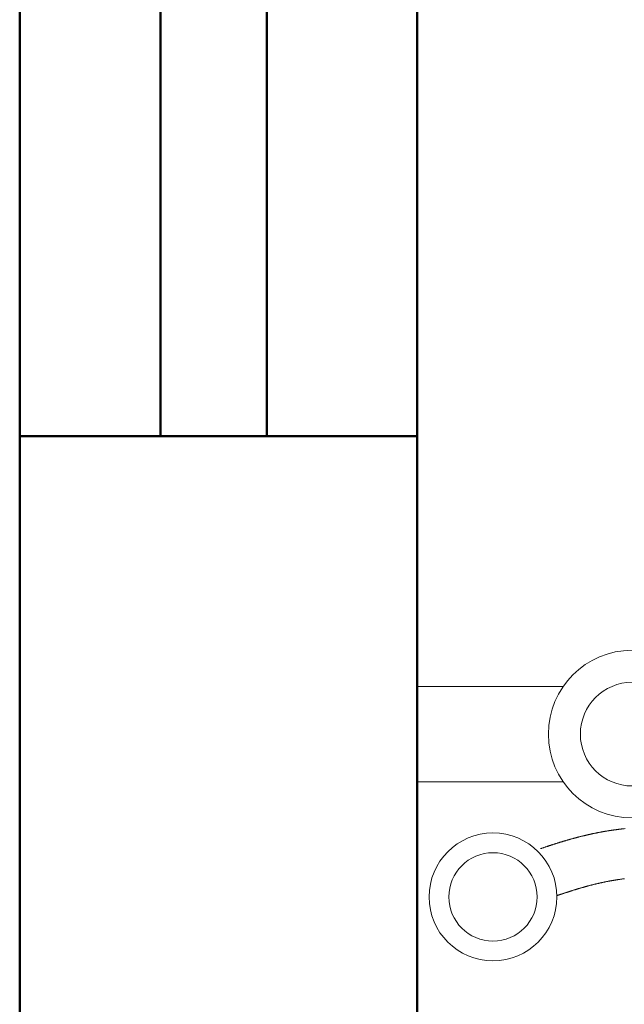
# Model space of a CAD drawing. Units: inches. Extents: x 64 to 1167, y 117 to 939.
# Tile 22 of 56: x 373.107 to 379.191, y 817.597 to 827.498. Entities that reach past the tile are written whole.
import ezdxf

# ---------------------------------------------------------------- set-up
doc = ezdxf.new("R2010")
doc.units = ezdxf.units.IN
doc.header["$MEASUREMENT"] = 0
doc.layers.add('A-FLOR-FIXT', color=8, linetype='Continuous', lineweight=18)
doc.layers.add('A-WALL', color=7, linetype='Continuous', lineweight=50)

# ---------------------------------------------------------------- blocks, each defined once
blk = doc.blocks.new('FAUCET')
blk.add_lwpolyline([(1.4695, 2.7601), (0.0003, 2.7601), (0.0003, 1.7995), (1.4695, 1.7995)])
for points in [[(2.0855, 0.8256, 0), (2.0364, 0.8191, 0), (1.9874, 0.8116, 0), (1.9385, 0.8031, 0), (1.8897, 0.7936, 0), (1.8409, 0.7831, 0), (1.7923, 0.7717, 0), (1.7437, 0.7595, 0), (1.6952, 0.7465, 0), (1.6468, 0.7328, 0), (1.5984, 0.7185, 0), (1.55, 0.7035, 0), (1.5018, 0.6879, 0), (1.4535, 0.6719, 0), (1.4054, 0.6555, 0)], [(2.0934, 1.3296, 0), (2.0807, 1.3283, 0), (2.068, 1.327, 0), (2.0553, 1.3255, 0), (2.0426, 1.3241, 0), (2.0299, 1.3226, 0), (2.0172, 1.321, 0), (2.0045, 1.3194, 0), (1.9917, 1.3177, 0), (1.979, 1.3159, 0), (1.9662, 1.3141, 0), (1.9535, 1.3123, 0), (1.9407, 1.3104, 0), (1.9279, 1.3084, 0), (1.9152, 1.3064, 0), (1.9024, 1.3043, 0), (1.8896, 1.3022, 0), (1.8769, 1.3, 0), (1.8642, 1.2977, 0), (1.8515, 1.2954, 0), (1.8388, 1.2931, 0), (1.8262, 1.2907, 0), (1.8136, 1.2882, 0), (1.801, 1.2857, 0), (1.7884, 1.2832, 0), (1.7759, 1.2806, 0), (1.7634, 1.2779, 0), (1.7509, 1.2752, 0), (1.7385, 1.2725, 0), (1.726, 1.2697, 0), (1.7137, 1.2669, 0), (1.7013, 1.264, 0), (1.689, 1.2611, 0), (1.6767, 1.2582, 0), (1.6644, 1.2552, 0), (1.6521, 1.2521, 0), (1.6399, 1.2491, 0), (1.6277, 1.246, 0), (1.6156, 1.2428, 0), (1.6034, 1.2396, 0), (1.5913, 1.2364, 0), (1.5792, 1.2332, 0), (1.5672, 1.2299, 0), (1.5552, 1.2266, 0), (1.5432, 1.2232, 0), (1.5312, 1.2199, 0), (1.5193, 1.2165, 0), (1.5074, 1.213, 0), (1.4955, 1.2096, 0), (1.4837, 1.2061, 0), (1.4719, 1.2026, 0), (1.4601, 1.199, 0), (1.4483, 1.1954, 0), (1.4366, 1.1919, 0), (1.4249, 1.1882, 0), (1.4133, 1.1846, 0), (1.4016, 1.181, 0), (1.39, 1.1773, 0), (1.3784, 1.1736, 0), (1.3669, 1.1699, 0), (1.3554, 1.1661, 0), (1.3439, 1.1624, 0), (1.3325, 1.1586, 0), (1.321, 1.1548, 0), (1.3097, 1.151, 0), (1.2983, 1.1472, 0), (1.287, 1.1434, 0), (1.2757, 1.1396, 0), (1.2644, 1.1357, 0), (1.2532, 1.1319, 0), (1.242, 1.128, 0)], [(2.0792, 1.3282, 0), (2.0747, 1.3277, 0), (2.0701, 1.3272, 0), (2.0655, 1.3267, 0), (2.0609, 1.3262, 0), (2.0563, 1.3257, 0), (2.0518, 1.3251, 0), (2.0472, 1.3246, 0), (2.0426, 1.3241, 0), (2.038, 1.3235, 0), (2.0334, 1.323, 0), (2.0288, 1.3224, 0), (2.0242, 1.3219, 0), (2.0197, 1.3213, 0), (2.0151, 1.3207, 0), (2.0105, 1.3201, 0), (2.0059, 1.3195, 0), (2.0013, 1.3189, 0), (1.9967, 1.3183, 0), (1.9921, 1.3177, 0), (1.9875, 1.3171, 0), (1.9829, 1.3165, 0), (1.9783, 1.3159, 0), (1.9737, 1.3152, 0), (1.9691, 1.3146, 0), (1.9645, 1.3139, 0), (1.9599, 1.3132, 0), (1.9553, 1.3126, 0), (1.9507, 1.3119, 0), (1.9461, 1.3112, 0), (1.9415, 1.3105, 0), (1.9369, 1.3098, 0), (1.9323, 1.3091, 0), (1.9277, 1.3084, 0), (1.9231, 1.3077, 0), (1.9185, 1.3069, 0), (1.9139, 1.3062, 0), (1.9093, 1.3054, 0), (1.9047, 1.3047, 0), (1.9001, 1.3039, 0), (1.8955, 1.3032, 0), (1.8909, 1.3024, 0), (1.8863, 1.3016, 0), (1.8817, 1.3008, 0), (1.8771, 1.3, 0), (1.8725, 1.2992, 0), (1.8679, 1.2984, 0), (1.8633, 1.2976, 0), (1.8587, 1.2968, 0), (1.8541, 1.2959, 0), (1.8496, 1.2951, 0), (1.845, 1.2943, 0), (1.8404, 1.2934, 0), (1.8359, 1.2925, 0), (1.8313, 1.2917, 0), (1.8268, 1.2908, 0), (1.8222, 1.2899, 0), (1.8177, 1.289, 0), (1.8131, 1.2882, 0), (1.8086, 1.2873, 0), (1.804, 1.2863, 0), (1.7995, 1.2854, 0), (1.795, 1.2845, 0), (1.7904, 1.2836, 0), (1.7859, 1.2827, 0), (1.7814, 1.2817, 0), (1.7769, 1.2808, 0), (1.7724, 1.2798, 0), (1.7679, 1.2789, 0), (1.7634, 1.2779, 0), (1.7589, 1.277, 0), (1.7544, 1.276, 0), (1.7499, 1.275, 0), (1.7454, 1.274, 0), (1.7409, 1.273, 0), (1.7364, 1.272, 0), (1.7319, 1.271, 0), (1.7275, 1.27, 0), (1.723, 1.269, 0), (1.7185, 1.268, 0), (1.714, 1.267, 0), (1.7096, 1.266, 0), (1.7051, 1.2649, 0), (1.7007, 1.2639, 0), (1.6962, 1.2628, 0), (1.6918, 1.2618, 0), (1.6873, 1.2607, 0), (1.6829, 1.2597, 0), (1.6785, 1.2586, 0), (1.674, 1.2575, 0), (1.6696, 1.2564, 0), (1.6652, 1.2554, 0), (1.6607, 1.2543, 0), (1.6563, 1.2532, 0), (1.6519, 1.2521, 0), (1.6475, 1.251, 0), (1.6431, 1.2499, 0), (1.6387, 1.2488, 0), (1.6343, 1.2476, 0), (1.6299, 1.2465, 0), (1.6255, 1.2454, 0), (1.6211, 1.2443, 0), (1.6167, 1.2431, 0), (1.6124, 1.242, 0), (1.608, 1.2408, 0), (1.6036, 1.2397, 0), (1.5992, 1.2385, 0), (1.5949, 1.2374, 0), (1.5905, 1.2362, 0), (1.5862, 1.235, 0), (1.5818, 1.2339, 0), (1.5774, 1.2327, 0), (1.5731, 1.2315, 0), (1.5688, 1.2303, 0), (1.5644, 1.2291, 0), (1.5601, 1.2279, 0), (1.5558, 1.2267, 0), (1.5514, 1.2255, 0), (1.5471, 1.2243, 0), (1.5428, 1.2231, 0), (1.5385, 1.2219, 0), (1.5342, 1.2207, 0), (1.5298, 1.2195, 0), (1.5255, 1.2182, 0), (1.5212, 1.217, 0), (1.5169, 1.2158, 0), (1.5126, 1.2145, 0), (1.5084, 1.2133, 0), (1.5041, 1.2121, 0), (1.4998, 1.2108, 0), (1.4955, 1.2096, 0), (1.4912, 1.2083, 0), (1.487, 1.207, 0), (1.4827, 1.2058, 0), (1.4784, 1.2045, 0), (1.4742, 1.2032, 0), (1.4699, 1.202, 0), (1.4657, 1.2007, 0), (1.4614, 1.1994, 0), (1.4572, 1.1981, 0), (1.4529, 1.1969, 0), (1.4487, 1.1956, 0), (1.4445, 1.1943, 0), (1.4403, 1.193, 0), (1.436, 1.1917, 0), (1.4318, 1.1904, 0), (1.4276, 1.1891, 0), (1.4234, 1.1878, 0), (1.4192, 1.1865, 0), (1.415, 1.1851, 0), (1.4108, 1.1838, 0), (1.4066, 1.1825, 0), (1.4024, 1.1812, 0), (1.3982, 1.1799, 0), (1.394, 1.1785, 0), (1.3898, 1.1772, 0), (1.3856, 1.1759, 0), (1.3815, 1.1746, 0), (1.3773, 1.1732, 0), (1.3731, 1.1719, 0), (1.369, 1.1705, 0), (1.3648, 1.1692, 0), (1.3607, 1.1678, 0), (1.3565, 1.1665, 0), (1.3524, 1.1652, 0), (1.3482, 1.1638, 0), (1.3441, 1.1624, 0), (1.34, 1.1611, 0), (1.3358, 1.1597, 0), (1.3317, 1.1584, 0), (1.3276, 1.157, 0), (1.3235, 1.1556, 0), (1.3194, 1.1543, 0), (1.3153, 1.1529, 0), (1.3112, 1.1515, 0), (1.307, 1.1502, 0), (1.303, 1.1488, 0), (1.2989, 1.1474, 0), (1.2948, 1.146, 0), (1.2907, 1.1447, 0), (1.2866, 1.1433, 0), (1.2825, 1.1419, 0), (1.2785, 1.1405, 0), (1.2744, 1.1391, 0), (1.2703, 1.1378, 0), (1.2663, 1.1364, 0), (1.2622, 1.135, 0), (1.2582, 1.1336, 0), (1.2541, 1.1322, 0), (1.2501, 1.1308, 0), (1.246, 1.1294, 0), (1.242, 1.128, 0)], [(2.0843, 0.8255, 0), (2.0792, 0.8249, 0), (2.0742, 0.8242, 0), (2.0691, 0.8236, 0), (2.0641, 0.8229, 0), (2.059, 0.8222, 0), (2.054, 0.8216, 0), (2.049, 0.8209, 0), (2.0439, 0.8202, 0), (2.0389, 0.8194, 0), (2.0338, 0.8187, 0), (2.0288, 0.818, 0), (2.0238, 0.8173, 0), (2.0187, 0.8165, 0), (2.0137, 0.8157, 0), (2.0087, 0.815, 0), (2.0036, 0.8142, 0), (1.9986, 0.8134, 0), (1.9936, 0.8126, 0), (1.9885, 0.8118, 0), (1.9835, 0.8109, 0), (1.9785, 0.8101, 0), (1.9734, 0.8093, 0), (1.9684, 0.8084, 0), (1.9634, 0.8075, 0), (1.9583, 0.8067, 0), (1.9533, 0.8058, 0), (1.9483, 0.8049, 0), (1.9433, 0.8039, 0), (1.9383, 0.803, 0), (1.9332, 0.8021, 0), (1.9282, 0.8012, 0), (1.9232, 0.8002, 0), (1.9182, 0.7992, 0), (1.9132, 0.7983, 0), (1.9081, 0.7973, 0), (1.9031, 0.7963, 0), (1.8981, 0.7953, 0), (1.8931, 0.7943, 0), (1.8881, 0.7932, 0), (1.8831, 0.7922, 0), (1.8781, 0.7911, 0), (1.8731, 0.7901, 0), (1.868, 0.789, 0), (1.863, 0.788, 0), (1.858, 0.7869, 0), (1.853, 0.7858, 0), (1.848, 0.7847, 0), (1.843, 0.7836, 0), (1.838, 0.7824, 0), (1.833, 0.7813, 0), (1.828, 0.7802, 0), (1.823, 0.779, 0), (1.818, 0.7778, 0), (1.813, 0.7767, 0), (1.808, 0.7755, 0), (1.803, 0.7743, 0), (1.798, 0.7731, 0), (1.793, 0.7719, 0), (1.788, 0.7707, 0), (1.783, 0.7695, 0), (1.778, 0.7682, 0), (1.773, 0.767, 0), (1.768, 0.7657, 0), (1.7631, 0.7645, 0), (1.7581, 0.7632, 0), (1.7531, 0.7619, 0), (1.7481, 0.7607, 0), (1.7431, 0.7594, 0), (1.7381, 0.7581, 0), (1.7331, 0.7568, 0), (1.7281, 0.7554, 0), (1.7232, 0.7541, 0), (1.7182, 0.7528, 0), (1.7132, 0.7514, 0), (1.7082, 0.7501, 0), (1.7032, 0.7487, 0), (1.6982, 0.7474, 0), (1.6933, 0.746, 0), (1.6883, 0.7446, 0), (1.6833, 0.7432, 0), (1.6783, 0.7418, 0), (1.6733, 0.7404, 0), (1.6684, 0.739, 0), (1.6634, 0.7376, 0), (1.6584, 0.7362, 0), (1.6534, 0.7348, 0), (1.6485, 0.7333, 0), (1.6435, 0.7319, 0), (1.6385, 0.7304, 0), (1.6335, 0.729, 0), (1.6286, 0.7275, 0), (1.6236, 0.726, 0), (1.6186, 0.7245, 0), (1.6136, 0.7231, 0), (1.6087, 0.7216, 0), (1.6037, 0.7201, 0), (1.5987, 0.7186, 0), (1.5938, 0.7171, 0), (1.5888, 0.7155, 0), (1.5838, 0.714, 0), (1.5789, 0.7125, 0), (1.5739, 0.7109, 0), (1.5689, 0.7094, 0), (1.564, 0.7078, 0), (1.559, 0.7063, 0), (1.554, 0.7047, 0), (1.5491, 0.7032, 0), (1.5441, 0.7016, 0), (1.5392, 0.7, 0), (1.5342, 0.6984, 0), (1.5292, 0.6968, 0), (1.5243, 0.6952, 0), (1.5193, 0.6936, 0), (1.5144, 0.692, 0), (1.5094, 0.6904, 0), (1.5044, 0.6888, 0), (1.4995, 0.6872, 0), (1.4945, 0.6856, 0), (1.4896, 0.6839, 0), (1.4846, 0.6823, 0), (1.4796, 0.6807, 0), (1.4747, 0.679, 0), (1.4697, 0.6774, 0), (1.4648, 0.6757, 0), (1.4598, 0.674, 0), (1.4549, 0.6724, 0), (1.4499, 0.6707, 0), (1.445, 0.669, 0), (1.44, 0.6673, 0), (1.4351, 0.6657, 0), (1.4301, 0.664, 0), (1.4252, 0.6623, 0), (1.4202, 0.6606, 0), (1.4153, 0.6589, 0), (1.4103, 0.6572, 0), (1.4054, 0.6555, 0)], [(2.0843, 0.8255, 0), (2.0792, 0.8249, 0), (2.0742, 0.8242, 0), (2.0691, 0.8236, 0), (2.0641, 0.8229, 0), (2.059, 0.8222, 0), (2.054, 0.8216, 0), (2.049, 0.8209, 0), (2.0439, 0.8202, 0), (2.0389, 0.8194, 0), (2.0338, 0.8187, 0), (2.0288, 0.818, 0), (2.0238, 0.8173, 0), (2.0187, 0.8165, 0), (2.0137, 0.8157, 0), (2.0087, 0.815, 0), (2.0036, 0.8142, 0), (1.9986, 0.8134, 0), (1.9936, 0.8126, 0), (1.9885, 0.8118, 0), (1.9835, 0.8109, 0), (1.9785, 0.8101, 0), (1.9734, 0.8093, 0), (1.9684, 0.8084, 0), (1.9634, 0.8075, 0), (1.9583, 0.8067, 0), (1.9533, 0.8058, 0), (1.9483, 0.8049, 0), (1.9433, 0.8039, 0), (1.9383, 0.803, 0), (1.9332, 0.8021, 0), (1.9282, 0.8012, 0), (1.9232, 0.8002, 0), (1.9182, 0.7992, 0), (1.9132, 0.7983, 0), (1.9081, 0.7973, 0), (1.9031, 0.7963, 0), (1.8981, 0.7953, 0), (1.8931, 0.7943, 0), (1.8881, 0.7932, 0), (1.8831, 0.7922, 0), (1.8781, 0.7911, 0), (1.8731, 0.7901, 0), (1.868, 0.789, 0), (1.863, 0.788, 0), (1.858, 0.7869, 0), (1.853, 0.7858, 0), (1.848, 0.7847, 0), (1.843, 0.7836, 0), (1.838, 0.7824, 0), (1.833, 0.7813, 0), (1.828, 0.7802, 0), (1.823, 0.779, 0), (1.818, 0.7778, 0), (1.813, 0.7767, 0), (1.808, 0.7755, 0), (1.803, 0.7743, 0), (1.798, 0.7731, 0), (1.793, 0.7719, 0), (1.788, 0.7707, 0), (1.783, 0.7695, 0), (1.778, 0.7682, 0), (1.773, 0.767, 0), (1.768, 0.7657, 0), (1.7631, 0.7645, 0), (1.7581, 0.7632, 0), (1.7531, 0.7619, 0), (1.7481, 0.7607, 0), (1.7431, 0.7594, 0), (1.7381, 0.7581, 0), (1.7331, 0.7568, 0), (1.7281, 0.7554, 0), (1.7232, 0.7541, 0), (1.7182, 0.7528, 0), (1.7132, 0.7514, 0), (1.7082, 0.7501, 0), (1.7032, 0.7487, 0), (1.6982, 0.7474, 0), (1.6933, 0.746, 0), (1.6883, 0.7446, 0), (1.6833, 0.7432, 0), (1.6783, 0.7418, 0), (1.6733, 0.7404, 0), (1.6684, 0.739, 0), (1.6634, 0.7376, 0), (1.6584, 0.7362, 0), (1.6534, 0.7348, 0), (1.6485, 0.7333, 0), (1.6435, 0.7319, 0), (1.6385, 0.7304, 0), (1.6335, 0.729, 0), (1.6286, 0.7275, 0), (1.6236, 0.726, 0), (1.6186, 0.7245, 0), (1.6136, 0.7231, 0), (1.6087, 0.7216, 0), (1.6037, 0.7201, 0), (1.5987, 0.7186, 0), (1.5938, 0.7171, 0), (1.5888, 0.7155, 0), (1.5838, 0.714, 0), (1.5789, 0.7125, 0), (1.5739, 0.7109, 0), (1.5689, 0.7094, 0), (1.564, 0.7078, 0), (1.559, 0.7063, 0), (1.554, 0.7047, 0), (1.5491, 0.7032, 0), (1.5441, 0.7016, 0), (1.5392, 0.7, 0), (1.5342, 0.6984, 0), (1.5292, 0.6968, 0), (1.5243, 0.6952, 0), (1.5193, 0.6936, 0), (1.5144, 0.692, 0), (1.5094, 0.6904, 0), (1.5044, 0.6888, 0), (1.4995, 0.6872, 0), (1.4945, 0.6856, 0), (1.4896, 0.6839, 0), (1.4846, 0.6823, 0), (1.4796, 0.6807, 0), (1.4747, 0.679, 0), (1.4697, 0.6774, 0), (1.4648, 0.6757, 0), (1.4598, 0.674, 0), (1.4549, 0.6724, 0), (1.4499, 0.6707, 0), (1.445, 0.669, 0), (1.44, 0.6673, 0), (1.4351, 0.6657, 0), (1.4301, 0.664, 0), (1.4252, 0.6623, 0), (1.4202, 0.6606, 0), (1.4153, 0.6589, 0), (1.4103, 0.6572, 0), (1.4054, 0.6555, 0)]]:
    blk.add_polyline3d(points)
for centre, radius in [((2.1627, 2.2798), 0.8433), ((2.1627, 2.2798), 0.5212), ((0.7624, 0.6428), 0.6431), ((0.7624, 0.6428), 0.4442)]:
    blk.add_circle(centre, radius)

msp = doc.modelspace()

# ---------------------------------------------------------------- linework, layer by layer
at = {"layer": 'A-WALL'}
for p, q in [((377.1073, 857.1998), (377.1073, 823.3109)), ((373.1073, 847.3109), (373.1073, 785.1998)), ((374.5241, 847.3109), (374.5241, 823.3109)), ((375.595, 847.3109), (375.595, 823.3109)), ((377.1073, 847.3109), (377.1073, 785.1998)), ((373.1073, 823.3109), (377.1073, 823.3109))]:
    msp.add_line(p, q, dxfattribs=at)

# ---------------------------------------------------------------- block references
at = {"layer": 'A-FLOR-FIXT'}
msp.add_blockref('FAUCET', (377.107, 818.034), dxfattribs=at)

doc.saveas('drawing.dxf')
